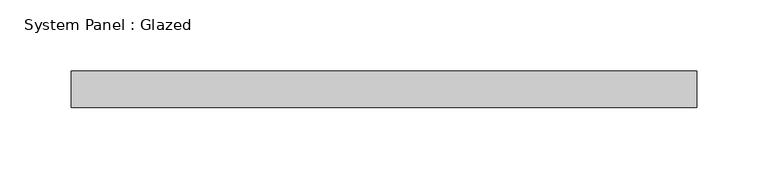
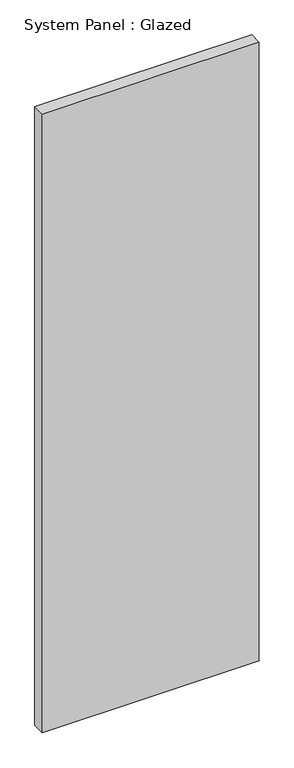
"""IFC4 building model written with IfcOpenShell, lengths in millimetres: plate geometry, System Panel : Glazed."""

from ifc_helpers import new_model, si_unit, origin, origin_with_axes, place, context, project, spatial, polyline, outline, extrude, source, transform, mapped, element, save


def system_panel_glazed_12bad0c7(model_context):
    return source(origin(), model_context, "Body", "SweptSolid", [
        extrude(outline(polyline([(219.075, 19.05), (-219.075, 19.05), (-219.075, 44.45), (219.075, 44.45), (219.075, 19.05)])), origin_with_axes(), (0.0, 0.0, 1.0), 1320.0507887),
    ])


if __name__ == "__main__":
    model = new_model("IFC4")
    model_context = context("Model", 3, world=origin())
    ifc_project = project(units=[si_unit("LENGTHUNIT", "METRE", prefix="MILLI")], contexts=[model_context])
    site = spatial("IfcSite", under=ifc_project)
    building = spatial("IfcBuilding", under=site)
    placement = place(None, origin())
    system_panel_glazed_shape = system_panel_glazed_12bad0c7(model_context)
    element("IfcPlate", 1, ObjectType="System Panel : Glazed", at=placement, inside=building, context=model_context, shape_type="MappedRepresentation", body=[
        mapped(system_panel_glazed_shape, transform((0.0, 0.0, 0.0), x_axis=(1.0, 0.0, 0.0), y_axis=(0.0, 1.0, 0.0), z_axis=(0.0, 0.0, 1.0))),
    ])
    save(model, "model.ifc")

# Revit data of these elements
# Type "System Panel : Glazed"
#   Construction Type Id = "GSP4R"
#   Analytic Construction = "1/8 in Pilkington single glazing"
#   Visual Light Transmittance = 0.9
#   Solar Heat Gain Coefficient = 0.86
#   Heat Transfer Coefficient (U) = 1.18115 BTU/(h·ft²·°F)
#   Define Thermal Properties by = 1
# Element 1 (IfcPlate, "System Panel : Glazed")
#   Materials on its faces: "Glass"
# Materials
#   "Glass": class "Glass", colour RGB 0 128 192, transparency 0.75, Description = "Soda Lime Glass", Cost = 0
